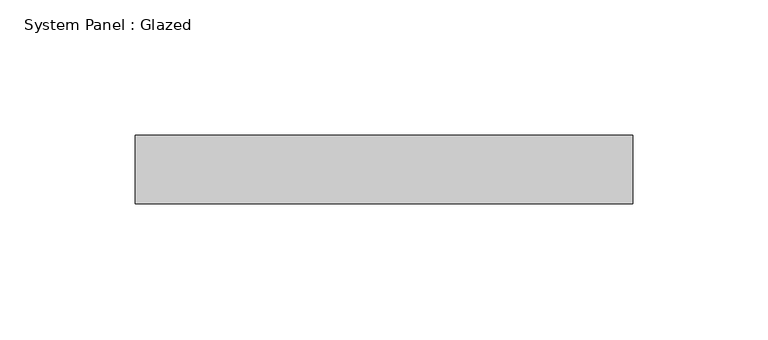
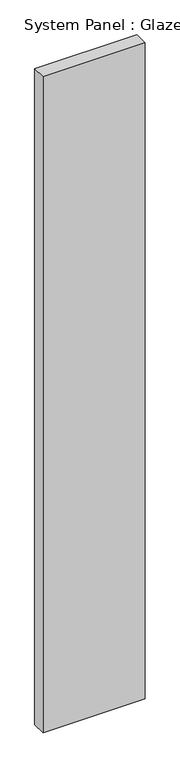
"""IFC4 building model written with IfcOpenShell, lengths in millimetres: plate geometry, System Panel : Glazed."""

from ifc_helpers import new_model, si_unit, origin, origin_with_axes, place, context, project, spatial, polyline, outline, extrude, source, transform, mapped, element, save


def system_panel_glazed_e70e5af4(model_context):
    return source(origin(), model_context, "Body", "SweptSolid", [
        extrude(outline(polyline([(92.075, 19.05), (-92.075, 19.05), (-92.075, 44.45), (92.075, 44.45), (92.075, 19.05)])), origin_with_axes(), (0.0, 0.0, 1.0), 1249.6336497),
    ])


if __name__ == "__main__":
    model = new_model("IFC4")
    model_context = context("Model", 3, world=origin())
    ifc_project = project(units=[si_unit("LENGTHUNIT", "METRE", prefix="MILLI")], contexts=[model_context])
    site = spatial("IfcSite", under=ifc_project)
    building = spatial("IfcBuilding", under=site)
    placement = place(None, origin())
    system_panel_glazed_shape = system_panel_glazed_e70e5af4(model_context)
    element("IfcPlate", 1, ObjectType="System Panel : Glazed", at=placement, inside=building, context=model_context, shape_type="MappedRepresentation", body=[
        mapped(system_panel_glazed_shape, transform((0.0, 0.0, 0.0), x_axis=(1.0, 0.0, 0.0), y_axis=(0.0, 1.0, 0.0), z_axis=(0.0, 0.0, 1.0))),
    ])
    save(model, "model.ifc")

# Revit data of these elements
# Type "System Panel : Glazed"
#   Construction Type Id = "GSP4R"
#   Analytic Construction = "1/8 in Pilkington single glazing"
#   Visual Light Transmittance = 0.9
#   Solar Heat Gain Coefficient = 0.86
#   Heat Transfer Coefficient (U) = 1.18115 BTU/(h·ft²·°F)
#   Define Thermal Properties by = 1
# Element 1 (IfcPlate, "System Panel : Glazed")
#   Materials on its faces: "Glass"
# Materials
#   "Glass": class "Glass", colour RGB 0 128 192, transparency 0.75, Description = "Soda Lime Glass", Cost = 0
